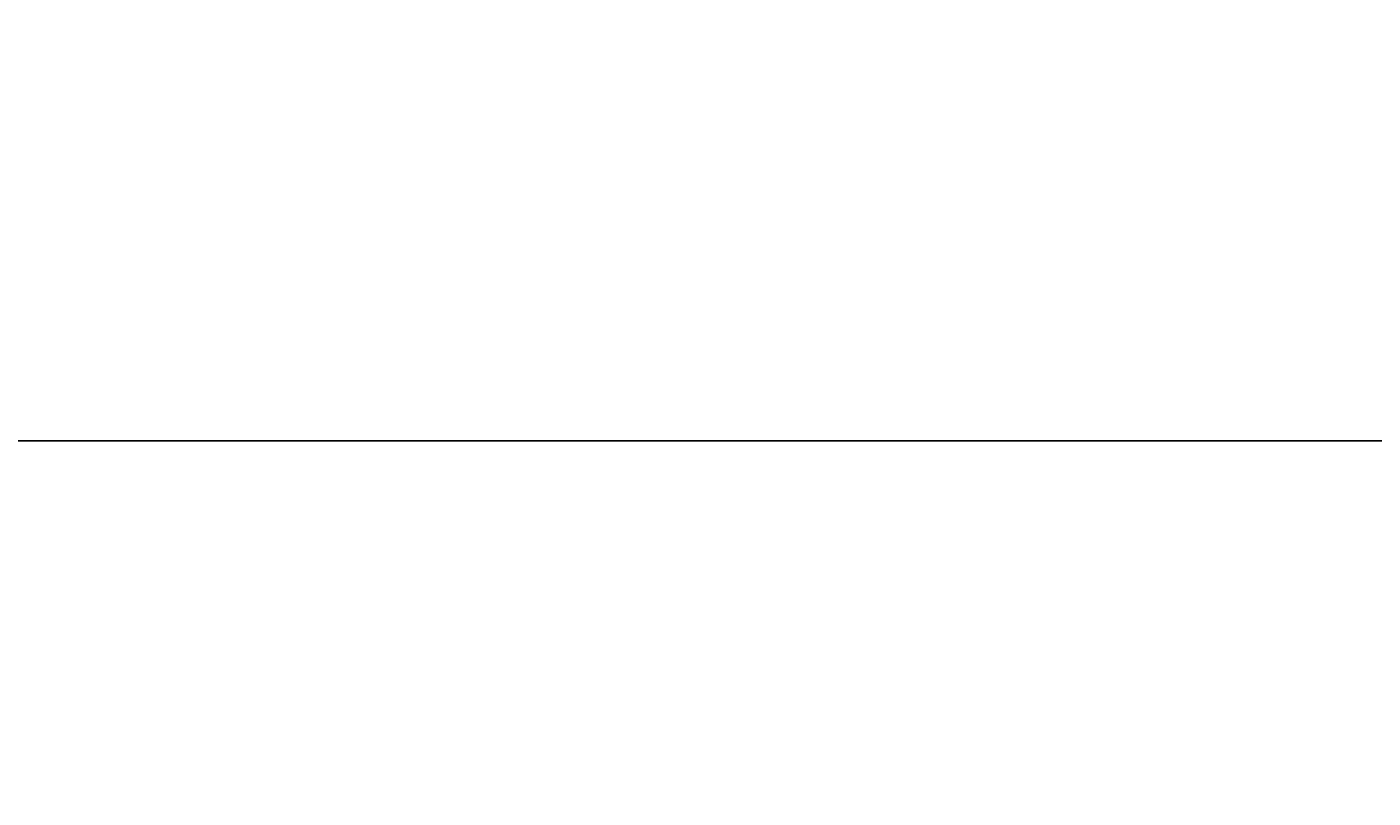
# Model space of a CAD drawing. Units: inches. Extents: x 84 to 1044, y -280 to 906.
# Tile 34 of 105: x 848 to 876, y -129 to -113. Entities that reach past the tile are written whole.
import ezdxf

# ---------------------------------------------------------------- set-up
doc = ezdxf.new("R2010")
doc.units = ezdxf.units.IN
doc.layers.add('A-ANNO-DIMS', color=2, linetype='Continuous', lineweight=18)
doc.layers.add('C-PROP', color=7, linetype='Continuous', lineweight=25)
doc.styles.get("Standard").update_dxf_attribs({"font": 'arial.ttf'})
doc.dimstyles.get("Standard").update_dxf_attribs({"dimtxt": 0.18, "dimasz": 0.18, "dimexe": 0.18, "dimexo": 0.0625, "dimgap": 0.09, "dimtad": 0, "dimtih": 1, "dimtoh": 1, "dimdec": 4, "dimzin": 0, "dimdsep": 46, "dimtxsty": 'Standard', "dimcen": 0.09, "dimadec": 0, "dimazin": 0, "dimtfac": 1, "dimtdec": 4, "dimtofl": 0, "dimtmove": 0, "dimatfit": 3, "dimfxl": 1, "dimtolj": 1, "dimtzin": 0, "dimarcsym": 0})

# ---------------------------------------------------------------- blocks, each defined once
blk = doc.blocks.new('*D60')
at = {"layer": 'A-ANNO-DIMS', "color": 0, "lineweight": -2, "transparency": 16777216}
for p, q in [((134.179, -121.942), (134.179, -180.64)), ((992.074, -121.942), (992.074, -180.64)), ((134.359, -180.46), (562.733, -180.46)), ((991.894, -180.46), (563.521, -180.46))]:
    blk.add_line(p, q, dxfattribs=at)
at = {"layer": 'A-ANNO-DIMS', "color": 0, "transparency": 16777216}
for points in [[(134.359, -180.43), (134.359, -180.49), (134.179, -180.46)], [(991.894, -180.43), (991.894, -180.49), (992.074, -180.46)]]:
    blk.add_solid(points, dxfattribs=at)
at = {"layer": 'Defpoints', "color": 0, "transparency": 16777216}
for p in [(134.179, -121.88), (992.074, -121.88), (992.074, -180.46)]:
    blk.add_point(p, dxfattribs=at)
at = {"layer": 'A-ANNO-DIMS', "color": 0, "transparency": 16777216, "insert": (563.127, -180.46), "char_height": 0.18, "attachment_point": 5}
blk.add_mtext('\\A1;857.9', dxfattribs=at)

msp = doc.modelspace()

# ---------------------------------------------------------------- linework, layer by layer
at = {"layer": 'C-PROP'}
msp.add_lwpolyline([(143.179, -121.88), (134.179, -121.88), (134.179, 856.12), (992.074, 856.12), (992.074, -121.88), (624.574, -121.88)], dxfattribs=at)

# ---------------------------------------------------------------- dimensions: what is measured, and where the dimension line sits
at = {"layer": 'A-ANNO-DIMS'}
dim = msp.add_linear_dim(base=(992.074, -180.46), p1=(134.179, -121.88), p2=(992.074, -121.88), dimstyle='Standard', override={"dimdec": 1, "dimlfac": 1, "dimrnd": 0, "dimzin": 0, "dimdsep": 46, "dimlunit": 2}, dxfattribs=at)
dim.commit()
dim.dimension.update_dxf_attribs({"geometry": '*D60', "text_midpoint": (563.127, -180.46)})

doc.saveas('drawing.dxf')
